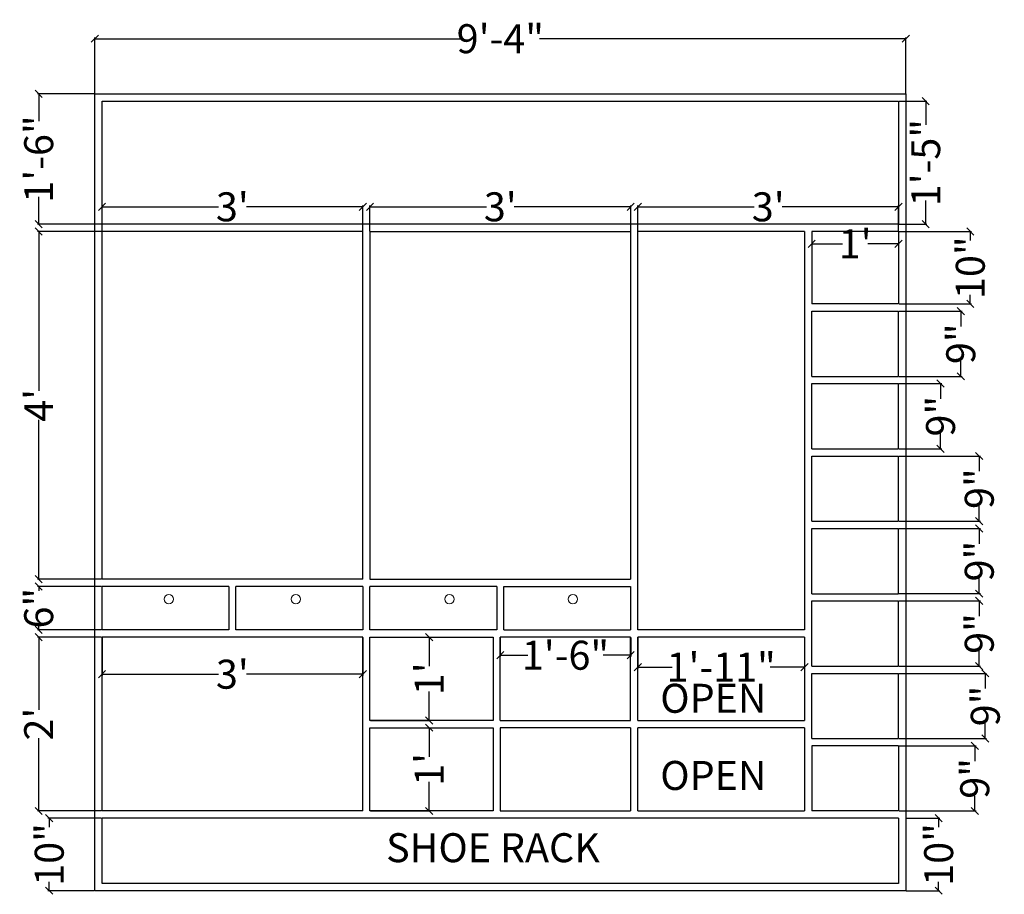
# Model space of a CAD drawing. Units: inches. Extents: x 221 to 357, y 425 to 545.
import ezdxf

# ---------------------------------------------------------------- set-up
doc = ezdxf.new("R2010")
doc.units = ezdxf.units.IN
doc.header["$MEASUREMENT"] = 0
for name, color, linetype, lineweight in [('A-ANNO-DIMS', 2, 'Continuous', 18), ('A-ANNO-TEXT', 3, 'Continuous', 18), ('A-FURN', 7, 'Continuous', 25), ('A-FURN-HDWR', 8, 'Continuous', 13)]:
    doc.layers.add(name, color=color, linetype=linetype, lineweight=lineweight)
doc.styles.get("Standard").update_dxf_attribs({"font": 'arial.ttf'})
doc.dimstyles.get("Standard").update_dxf_attribs({"dimtxt": 4, "dimasz": 1, "dimexe": 0.18, "dimexo": 0.0625, "dimgap": 0.09, "dimtad": 0, "dimdec": 4, "dimzin": 0, "dimdsep": 46, "dimlunit": 4, "dimtxsty": 'Standard', "dimblk": 'OBLIQUE', "dimcen": 0.09, "dimadec": 0, "dimazin": 0, "dimtfac": 1, "dimtdec": 4, "dimtofl": 0, "dimtmove": 0, "dimatfit": 3, "dimldrblk": 'OBLIQUE', "dimfxl": 1, "dimtolj": 1, "dimtzin": 0, "dimarcsym": 1})

# ---------------------------------------------------------------- blocks, each defined once
blk = doc.blocks.new('_Oblique')
at = {"color": 0, "linetype": 'ByBlock', "lineweight": -2}
blk.add_line((-0.5, -0.5), (0.5, 0.5), dxfattribs=at)
blk = doc.blocks.new('*D2')
at = {"layer": 'A-ANNO-DIMS', "color": 0, "lineweight": -2, "transparency": 16777216}
for p, q in [((342.92, 534.06), (346.78, 534.06)), ((346.6, 534.06), (346.6, 530.78)), ((346.6, 517.06), (346.6, 520.34)), ((342.92, 517.06), (346.78, 517.06))]:
    blk.add_line(p, q, dxfattribs=at)
at = {"layer": 'Defpoints', "color": 0, "transparency": 16777216}
for p in [(342.86, 534.06), (342.86, 517.06), (346.6, 517.06)]:
    blk.add_point(p, dxfattribs=at)
at = {"layer": 'A-ANNO-DIMS', "color": 0, "lineweight": -2, "transparency": 16777216}
for p, rotation in [((346.6, 534.06), 90), ((346.6, 517.06), 270)]:
    blk.add_blockref('_Oblique', p, dxfattribs=dict(at, rotation=rotation))
at = {"layer": 'A-ANNO-DIMS', "color": 0, "transparency": 16777216, "insert": (346.6, 525.56), "char_height": 4, "attachment_point": 5, "rotation": 90}
blk.add_mtext('\\A1;1\'-5"', dxfattribs=at)
blk = doc.blocks.new('*D3')
at = {"layer": 'A-ANNO-DIMS', "color": 0, "lineweight": -2, "transparency": 16777216}
for p, q in [((343.92, 435.06), (348.57, 435.06)), ((348.39, 435.06), (348.39, 433.81)), ((348.39, 425.06), (348.39, 426.3)), ((343.92, 425.06), (348.57, 425.06))]:
    blk.add_line(p, q, dxfattribs=at)
at = {"layer": 'Defpoints', "color": 0, "transparency": 16777216}
for p in [(343.86, 435.06), (348.39, 435.06), (343.86, 425.06)]:
    blk.add_point(p, dxfattribs=at)
at = {"layer": 'A-ANNO-DIMS', "color": 0, "lineweight": -2, "transparency": 16777216}
for p, rotation in [((348.39, 435.06), 90), ((348.39, 425.06), 270)]:
    blk.add_blockref('_Oblique', p, dxfattribs=dict(at, rotation=rotation))
at = {"layer": 'A-ANNO-DIMS', "color": 0, "transparency": 16777216, "insert": (348.39, 430.06), "char_height": 4, "attachment_point": 5, "rotation": 90}
blk.add_mtext('\\A1;10"', dxfattribs=at)
blk = doc.blocks.new('*D4')
at = {"layer": 'A-ANNO-DIMS', "color": 0, "lineweight": -2, "transparency": 16777216}
for p, q in [((342.92, 516.06), (352.94, 516.06)), ((352.76, 516.06), (352.76, 514.81)), ((352.76, 506.06), (352.76, 507.3)), ((342.92, 506.06), (352.94, 506.06))]:
    blk.add_line(p, q, dxfattribs=at)
at = {"layer": 'Defpoints', "color": 0, "transparency": 16777216}
for p in [(342.86, 516.06), (342.86, 506.06), (352.76, 506.06)]:
    blk.add_point(p, dxfattribs=at)
at = {"layer": 'A-ANNO-DIMS', "color": 0, "lineweight": -2, "transparency": 16777216}
for p, rotation in [((352.76, 516.06), 90), ((352.76, 506.06), 270)]:
    blk.add_blockref('_Oblique', p, dxfattribs=dict(at, rotation=rotation))
at = {"layer": 'A-ANNO-DIMS', "color": 0, "transparency": 16777216, "insert": (352.76, 511.06), "char_height": 4, "attachment_point": 5, "rotation": 90}
blk.add_mtext('\\A1;10"', dxfattribs=at)
blk = doc.blocks.new('*D5')
at = {"layer": 'A-ANNO-DIMS', "color": 0, "lineweight": -2, "transparency": 16777216}
for p, q in [((342.92, 505.06), (351.62, 505.06)), ((351.44, 505.06), (351.44, 502.95)), ((351.44, 496.06), (351.44, 498.17)), ((342.92, 496.06), (351.62, 496.06))]:
    blk.add_line(p, q, dxfattribs=at)
at = {"layer": 'Defpoints', "color": 0, "transparency": 16777216}
for p in [(342.86, 505.06), (342.86, 496.06), (351.44, 496.06)]:
    blk.add_point(p, dxfattribs=at)
at = {"layer": 'A-ANNO-DIMS', "color": 0, "lineweight": -2, "transparency": 16777216}
for p, rotation in [((351.44, 505.06), 90), ((351.44, 496.06), 270)]:
    blk.add_blockref('_Oblique', p, dxfattribs=dict(at, rotation=rotation))
at = {"layer": 'A-ANNO-DIMS', "color": 0, "transparency": 16777216, "insert": (351.44, 500.56), "char_height": 4, "attachment_point": 5, "rotation": 90}
blk.add_mtext('\\A1;9"', dxfattribs=at)
blk = doc.blocks.new('*D6')
at = {"layer": 'A-ANNO-DIMS', "color": 0, "lineweight": -2, "transparency": 16777216}
for p, q in [((342.92, 495.06), (348.83, 495.06)), ((348.65, 495.06), (348.65, 492.95)), ((348.65, 486.06), (348.65, 488.17)), ((342.92, 486.06), (348.83, 486.06))]:
    blk.add_line(p, q, dxfattribs=at)
at = {"layer": 'Defpoints', "color": 0, "transparency": 16777216}
for p in [(342.86, 495.06), (342.86, 486.06), (348.65, 486.06)]:
    blk.add_point(p, dxfattribs=at)
at = {"layer": 'A-ANNO-DIMS', "color": 0, "lineweight": -2, "transparency": 16777216}
for p, rotation in [((348.65, 495.06), 90), ((348.65, 486.06), 270)]:
    blk.add_blockref('_Oblique', p, dxfattribs=dict(at, rotation=rotation))
at = {"layer": 'A-ANNO-DIMS', "color": 0, "transparency": 16777216, "insert": (348.65, 490.56), "char_height": 4, "attachment_point": 5, "rotation": 90}
blk.add_mtext('\\A1;9"', dxfattribs=at)
blk = doc.blocks.new('*D7')
at = {"layer": 'A-ANNO-DIMS', "color": 0, "lineweight": -2, "transparency": 16777216}
for p, q in [((342.92, 485.06), (354.18, 485.06)), ((354, 485.06), (354, 482.95)), ((354, 476.06), (354, 478.17)), ((342.92, 476.06), (354.18, 476.06))]:
    blk.add_line(p, q, dxfattribs=at)
at = {"layer": 'Defpoints', "color": 0, "transparency": 16777216}
for p in [(342.86, 485.06), (342.86, 476.06), (354, 476.06)]:
    blk.add_point(p, dxfattribs=at)
at = {"layer": 'A-ANNO-DIMS', "color": 0, "lineweight": -2, "transparency": 16777216}
for p, rotation in [((354, 485.06), 90), ((354, 476.06), 270)]:
    blk.add_blockref('_Oblique', p, dxfattribs=dict(at, rotation=rotation))
at = {"layer": 'A-ANNO-DIMS', "color": 0, "transparency": 16777216, "insert": (354, 480.56), "char_height": 4, "attachment_point": 5, "rotation": 90}
blk.add_mtext('\\A1;9"', dxfattribs=at)
blk = doc.blocks.new('*D8')
at = {"layer": 'A-ANNO-DIMS', "color": 0, "lineweight": -2, "transparency": 16777216}
for p, q in [((342.92, 475.06), (354.18, 475.06)), ((354, 475.06), (354, 472.95)), ((354, 466.06), (354, 468.17)), ((342.92, 466.06), (354.18, 466.06))]:
    blk.add_line(p, q, dxfattribs=at)
at = {"layer": 'Defpoints', "color": 0, "transparency": 16777216}
for p in [(342.86, 475.06), (342.86, 466.06), (354, 466.06)]:
    blk.add_point(p, dxfattribs=at)
at = {"layer": 'A-ANNO-DIMS', "color": 0, "lineweight": -2, "transparency": 16777216}
for p, rotation in [((354, 475.06), 90), ((354, 466.06), 270)]:
    blk.add_blockref('_Oblique', p, dxfattribs=dict(at, rotation=rotation))
at = {"layer": 'A-ANNO-DIMS', "color": 0, "transparency": 16777216, "insert": (354, 470.56), "char_height": 4, "attachment_point": 5, "rotation": 90}
blk.add_mtext('\\A1;9"', dxfattribs=at)
blk = doc.blocks.new('*D9')
at = {"layer": 'A-ANNO-DIMS', "color": 0, "lineweight": -2, "transparency": 16777216}
for p, q in [((342.92, 465.06), (354.18, 465.06)), ((354, 465.06), (354, 462.95)), ((354, 456.06), (354, 458.17)), ((342.92, 456.06), (354.18, 456.06))]:
    blk.add_line(p, q, dxfattribs=at)
at = {"layer": 'Defpoints', "color": 0, "transparency": 16777216}
for p in [(342.86, 465.06), (342.86, 456.06), (354, 456.06)]:
    blk.add_point(p, dxfattribs=at)
at = {"layer": 'A-ANNO-DIMS', "color": 0, "lineweight": -2, "transparency": 16777216}
for p, rotation in [((354, 465.06), 90), ((354, 456.06), 270)]:
    blk.add_blockref('_Oblique', p, dxfattribs=dict(at, rotation=rotation))
at = {"layer": 'A-ANNO-DIMS', "color": 0, "transparency": 16777216, "insert": (354, 460.56), "char_height": 4, "attachment_point": 5, "rotation": 90}
blk.add_mtext('\\A1;9"', dxfattribs=at)
blk = doc.blocks.new('*D10')
at = {"layer": 'A-ANNO-DIMS', "color": 0, "lineweight": -2, "transparency": 16777216}
for p, q in [((342.92, 455.06), (355.01, 455.06)), ((354.83, 455.06), (354.83, 452.95)), ((354.83, 446.06), (354.83, 448.17)), ((342.92, 446.06), (355.01, 446.06))]:
    blk.add_line(p, q, dxfattribs=at)
at = {"layer": 'Defpoints', "color": 0, "transparency": 16777216}
for p in [(342.86, 455.06), (342.86, 446.06), (354.83, 446.06)]:
    blk.add_point(p, dxfattribs=at)
at = {"layer": 'A-ANNO-DIMS', "color": 0, "lineweight": -2, "transparency": 16777216}
for p, rotation in [((354.83, 455.06), 90), ((354.83, 446.06), 270)]:
    blk.add_blockref('_Oblique', p, dxfattribs=dict(at, rotation=rotation))
at = {"layer": 'A-ANNO-DIMS', "color": 0, "transparency": 16777216, "insert": (354.83, 450.56), "char_height": 4, "attachment_point": 5, "rotation": 90}
blk.add_mtext('\\A1;9"', dxfattribs=at)
blk = doc.blocks.new('*D11')
at = {"layer": 'A-ANNO-DIMS', "color": 0, "lineweight": -2, "transparency": 16777216}
for p, q in [((342.92, 445.06), (353.55, 445.06)), ((353.37, 445.06), (353.37, 442.95)), ((353.37, 436.06), (353.37, 438.17)), ((342.92, 436.06), (353.55, 436.06))]:
    blk.add_line(p, q, dxfattribs=at)
at = {"layer": 'Defpoints', "color": 0, "transparency": 16777216}
for p in [(342.86, 445.06), (342.86, 436.06), (353.37, 436.06)]:
    blk.add_point(p, dxfattribs=at)
at = {"layer": 'A-ANNO-DIMS', "color": 0, "lineweight": -2, "transparency": 16777216}
for p, rotation in [((353.37, 445.06), 90), ((353.37, 436.06), 270)]:
    blk.add_blockref('_Oblique', p, dxfattribs=dict(at, rotation=rotation))
at = {"layer": 'A-ANNO-DIMS', "color": 0, "transparency": 16777216, "insert": (353.37, 440.56), "char_height": 4, "attachment_point": 5, "rotation": 90}
blk.add_mtext('\\A1;9"', dxfattribs=at)
blk = doc.blocks.new('*D12')
at = {"layer": 'A-ANNO-DIMS', "color": 0, "lineweight": -2, "transparency": 16777216}
for p, q in [((306.86, 460), (306.86, 455.75)), ((329.86, 460), (329.86, 455.75)), ((306.86, 455.93), (311.58, 455.93)), ((329.86, 455.93), (325.13, 455.93))]:
    blk.add_line(p, q, dxfattribs=at)
at = {"layer": 'Defpoints', "color": 0, "transparency": 16777216}
for p in [(306.86, 460.06), (329.86, 460.06), (306.86, 455.93)]:
    blk.add_point(p, dxfattribs=at)
at = {"layer": 'A-ANNO-DIMS', "color": 0, "lineweight": -2, "transparency": 16777216, "rotation": 180}
blk.add_blockref('_Oblique', (306.86, 455.93), dxfattribs=at)
at = {"layer": 'A-ANNO-DIMS', "color": 0, "lineweight": -2, "transparency": 16777216}
blk.add_blockref('_Oblique', (329.86, 455.93), dxfattribs=at)
at = {"layer": 'A-ANNO-DIMS', "color": 0, "transparency": 16777216, "insert": (318.36, 455.93), "char_height": 4, "attachment_point": 5}
blk.add_mtext('\\A1;1\'-11"', dxfattribs=at)
blk = doc.blocks.new('*D13')
at = {"layer": 'A-ANNO-DIMS', "color": 0, "lineweight": -2, "transparency": 16777216}
for p, q in [((287.86, 460), (287.86, 457.38)), ((305.86, 460), (305.86, 457.38)), ((287.86, 457.56), (291.64, 457.56)), ((305.86, 457.56), (302.07, 457.56))]:
    blk.add_line(p, q, dxfattribs=at)
at = {"layer": 'Defpoints', "color": 0, "transparency": 16777216}
for p in [(287.86, 460.06), (305.86, 460.06), (287.86, 457.56)]:
    blk.add_point(p, dxfattribs=at)
at = {"layer": 'A-ANNO-DIMS', "color": 0, "lineweight": -2, "transparency": 16777216, "rotation": 180}
blk.add_blockref('_Oblique', (287.86, 457.56), dxfattribs=at)
at = {"layer": 'A-ANNO-DIMS', "color": 0, "lineweight": -2, "transparency": 16777216}
blk.add_blockref('_Oblique', (305.86, 457.56), dxfattribs=at)
at = {"layer": 'A-ANNO-DIMS', "color": 0, "transparency": 16777216, "insert": (296.86, 457.56), "char_height": 4, "attachment_point": 5}
blk.add_mtext('\\A1;1\'-6"', dxfattribs=at)
blk = doc.blocks.new('*D14')
at = {"layer": 'A-ANNO-DIMS', "color": 0, "lineweight": -2, "transparency": 16777216}
for p, q in [((269.92, 460.06), (278.21, 460.06)), ((278.03, 460.06), (278.03, 456.05)), ((278.03, 448.56), (278.03, 452.57)), ((269.92, 448.56), (278.21, 448.56))]:
    blk.add_line(p, q, dxfattribs=at)
at = {"layer": 'Defpoints', "color": 0, "transparency": 16777216}
for p in [(269.86, 460.06), (278.03, 460.06), (269.86, 448.56)]:
    blk.add_point(p, dxfattribs=at)
at = {"layer": 'A-ANNO-DIMS', "color": 0, "lineweight": -2, "transparency": 16777216}
for p, rotation in [((278.03, 460.06), 90), ((278.03, 448.56), 270)]:
    blk.add_blockref('_Oblique', p, dxfattribs=dict(at, rotation=rotation))
at = {"layer": 'A-ANNO-DIMS', "color": 0, "transparency": 16777216, "insert": (278.03, 454.31), "char_height": 4, "attachment_point": 5, "rotation": 90}
blk.add_mtext("\\A1;1'", dxfattribs=at)
blk = doc.blocks.new('*D15')
at = {"layer": 'A-ANNO-DIMS', "color": 0, "lineweight": -2, "transparency": 16777216}
for p, q in [((232.86, 460), (232.86, 454.76)), ((268.86, 460), (268.86, 454.76)), ((232.86, 454.94), (248.93, 454.94)), ((268.86, 454.94), (252.79, 454.94))]:
    blk.add_line(p, q, dxfattribs=at)
at = {"layer": 'Defpoints', "color": 0, "transparency": 16777216}
for p in [(232.86, 460.06), (268.86, 460.06), (232.86, 454.94)]:
    blk.add_point(p, dxfattribs=at)
at = {"layer": 'A-ANNO-DIMS', "color": 0, "lineweight": -2, "transparency": 16777216, "rotation": 180}
blk.add_blockref('_Oblique', (232.86, 454.94), dxfattribs=at)
at = {"layer": 'A-ANNO-DIMS', "color": 0, "lineweight": -2, "transparency": 16777216}
blk.add_blockref('_Oblique', (268.86, 454.94), dxfattribs=at)
at = {"layer": 'A-ANNO-DIMS', "color": 0, "transparency": 16777216, "insert": (250.86, 454.94), "char_height": 4, "attachment_point": 5}
blk.add_mtext("\\A1;3'", dxfattribs=at)
blk = doc.blocks.new('*D16')
at = {"layer": 'A-ANNO-DIMS', "color": 0, "lineweight": -2, "transparency": 16777216}
for p, q in [((232.86, 516.12), (232.86, 519.64)), ((232.86, 519.46), (248.93, 519.46)), ((268.86, 519.46), (252.79, 519.46)), ((268.86, 516.12), (268.86, 519.64))]:
    blk.add_line(p, q, dxfattribs=at)
at = {"layer": 'Defpoints', "color": 0, "transparency": 16777216}
for p in [(232.86, 519.46), (232.86, 516.06), (268.86, 516.06)]:
    blk.add_point(p, dxfattribs=at)
at = {"layer": 'A-ANNO-DIMS', "color": 0, "lineweight": -2, "transparency": 16777216, "rotation": 180}
blk.add_blockref('_Oblique', (232.86, 519.46), dxfattribs=at)
at = {"layer": 'A-ANNO-DIMS', "color": 0, "lineweight": -2, "transparency": 16777216}
blk.add_blockref('_Oblique', (268.86, 519.46), dxfattribs=at)
at = {"layer": 'A-ANNO-DIMS', "color": 0, "transparency": 16777216, "insert": (250.86, 519.46), "char_height": 4, "attachment_point": 5}
blk.add_mtext("\\A1;3'", dxfattribs=at)
blk = doc.blocks.new('*D17')
at = {"layer": 'A-ANNO-DIMS', "color": 0, "lineweight": -2, "transparency": 16777216}
for p, q in [((269.86, 516.12), (269.86, 519.64)), ((269.86, 519.46), (285.93, 519.46)), ((305.86, 519.46), (289.79, 519.46)), ((305.86, 516.12), (305.86, 519.64))]:
    blk.add_line(p, q, dxfattribs=at)
at = {"layer": 'Defpoints', "color": 0, "transparency": 16777216}
for p in [(269.86, 519.46), (269.86, 516.06), (305.86, 516.06)]:
    blk.add_point(p, dxfattribs=at)
at = {"layer": 'A-ANNO-DIMS', "color": 0, "lineweight": -2, "transparency": 16777216, "rotation": 180}
blk.add_blockref('_Oblique', (269.86, 519.46), dxfattribs=at)
at = {"layer": 'A-ANNO-DIMS', "color": 0, "lineweight": -2, "transparency": 16777216}
blk.add_blockref('_Oblique', (305.86, 519.46), dxfattribs=at)
at = {"layer": 'A-ANNO-DIMS', "color": 0, "transparency": 16777216, "insert": (287.86, 519.46), "char_height": 4, "attachment_point": 5}
blk.add_mtext("\\A1;3'", dxfattribs=at)
blk = doc.blocks.new('*D18')
at = {"layer": 'A-ANNO-DIMS', "color": 0, "lineweight": -2, "transparency": 16777216}
for p, q in [((306.86, 516.12), (306.86, 519.64)), ((306.86, 519.46), (322.93, 519.46)), ((342.86, 519.46), (326.79, 519.46)), ((342.86, 516.12), (342.86, 519.64))]:
    blk.add_line(p, q, dxfattribs=at)
at = {"layer": 'Defpoints', "color": 0, "transparency": 16777216}
for p in [(342.86, 519.46), (306.86, 516.06), (342.86, 516.06)]:
    blk.add_point(p, dxfattribs=at)
at = {"layer": 'A-ANNO-DIMS', "color": 0, "lineweight": -2, "transparency": 16777216, "rotation": 180}
blk.add_blockref('_Oblique', (306.86, 519.46), dxfattribs=at)
at = {"layer": 'A-ANNO-DIMS', "color": 0, "lineweight": -2, "transparency": 16777216}
blk.add_blockref('_Oblique', (342.86, 519.46), dxfattribs=at)
at = {"layer": 'A-ANNO-DIMS', "color": 0, "transparency": 16777216, "insert": (324.86, 519.46), "char_height": 4, "attachment_point": 5}
blk.add_mtext("\\A1;3'", dxfattribs=at)
blk = doc.blocks.new('*D19')
at = {"layer": 'A-ANNO-DIMS', "color": 0, "lineweight": -2, "transparency": 16777216}
for p, q in [((330.86, 516), (330.86, 514.18)), ((342.86, 516), (342.86, 514.18)), ((330.86, 514.36), (335.11, 514.36)), ((342.86, 514.36), (338.6, 514.36))]:
    blk.add_line(p, q, dxfattribs=at)
at = {"layer": 'Defpoints', "color": 0, "transparency": 16777216}
for p in [(330.86, 516.06), (342.86, 516.06), (330.86, 514.36)]:
    blk.add_point(p, dxfattribs=at)
at = {"layer": 'A-ANNO-DIMS', "color": 0, "lineweight": -2, "transparency": 16777216, "rotation": 180}
blk.add_blockref('_Oblique', (330.86, 514.36), dxfattribs=at)
at = {"layer": 'A-ANNO-DIMS', "color": 0, "lineweight": -2, "transparency": 16777216}
blk.add_blockref('_Oblique', (342.86, 514.36), dxfattribs=at)
at = {"layer": 'A-ANNO-DIMS', "color": 0, "transparency": 16777216, "insert": (336.86, 514.36), "char_height": 4, "attachment_point": 5}
blk.add_mtext("\\A1;1'", dxfattribs=at)
blk = doc.blocks.new('*D20')
at = {"layer": 'A-ANNO-DIMS', "color": 0, "lineweight": -2, "transparency": 16777216}
for p, q in [((269.92, 447.56), (278.21, 447.56)), ((278.03, 447.56), (278.03, 443.55)), ((278.03, 436.06), (278.03, 440.07)), ((269.92, 436.06), (278.21, 436.06))]:
    blk.add_line(p, q, dxfattribs=at)
at = {"layer": 'Defpoints', "color": 0, "transparency": 16777216}
for p in [(269.86, 447.56), (278.03, 447.56), (269.86, 436.06)]:
    blk.add_point(p, dxfattribs=at)
at = {"layer": 'A-ANNO-DIMS', "color": 0, "lineweight": -2, "transparency": 16777216}
for p, rotation in [((278.03, 447.56), 90), ((278.03, 436.06), 270)]:
    blk.add_blockref('_Oblique', p, dxfattribs=dict(at, rotation=rotation))
at = {"layer": 'A-ANNO-DIMS', "color": 0, "transparency": 16777216, "insert": (278.03, 441.81), "char_height": 4, "attachment_point": 5, "rotation": 90}
blk.add_mtext("\\A1;1'", dxfattribs=at)
blk = doc.blocks.new('*D21')
at = {"layer": 'A-ANNO-DIMS', "color": 0, "lineweight": -2, "transparency": 16777216}
for p, q in [((232.79, 435.06), (225.39, 435.06)), ((225.57, 435.06), (225.57, 433.81)), ((225.57, 425.06), (225.57, 426.3)), ((231.79, 425.06), (225.39, 425.06))]:
    blk.add_line(p, q, dxfattribs=at)
at = {"layer": 'Defpoints', "color": 0, "transparency": 16777216}
for p in [(225.57, 435.06), (232.86, 435.06), (231.86, 425.06)]:
    blk.add_point(p, dxfattribs=at)
at = {"layer": 'A-ANNO-DIMS', "color": 0, "lineweight": -2, "transparency": 16777216}
for p, rotation in [((225.57, 435.06), 90), ((225.57, 425.06), 270)]:
    blk.add_blockref('_Oblique', p, dxfattribs=dict(at, rotation=rotation))
at = {"layer": 'A-ANNO-DIMS', "color": 0, "transparency": 16777216, "insert": (225.57, 430.06), "char_height": 4, "attachment_point": 5, "rotation": 90}
blk.add_mtext('\\A1;10"', dxfattribs=at)
blk = doc.blocks.new('*D22')
at = {"layer": 'A-ANNO-DIMS', "color": 0, "lineweight": -2, "transparency": 16777216}
for p, q in [((232.79, 460.06), (223.93, 460.06)), ((224.11, 460.06), (224.11, 450.02)), ((224.11, 436.06), (224.11, 446.09)), ((232.79, 436.06), (223.93, 436.06))]:
    blk.add_line(p, q, dxfattribs=at)
at = {"layer": 'Defpoints', "color": 0, "transparency": 16777216}
for p in [(224.11, 460.06), (232.86, 460.06), (232.86, 436.06)]:
    blk.add_point(p, dxfattribs=at)
at = {"layer": 'A-ANNO-DIMS', "color": 0, "lineweight": -2, "transparency": 16777216}
for p, rotation in [((224.11, 460.06), 90), ((224.11, 436.06), 270)]:
    blk.add_blockref('_Oblique', p, dxfattribs=dict(at, rotation=rotation))
at = {"layer": 'A-ANNO-DIMS', "color": 0, "transparency": 16777216, "insert": (224.11, 448.06), "char_height": 4, "attachment_point": 5, "rotation": 90}
blk.add_mtext("\\A1;2'", dxfattribs=at)
blk = doc.blocks.new('*D23')
at = {"layer": 'A-ANNO-DIMS', "color": 0, "lineweight": -2, "transparency": 16777216}
for p, q in [((232.79, 467.06), (223.93, 467.06)), ((224.11, 467.06), (224.11, 466.46)), ((232.79, 461.06), (223.93, 461.06)), ((224.11, 461.06), (224.11, 461.66))]:
    blk.add_line(p, q, dxfattribs=at)
at = {"layer": 'Defpoints', "color": 0, "transparency": 16777216}
for p in [(224.11, 467.06), (232.86, 467.06), (232.86, 461.06)]:
    blk.add_point(p, dxfattribs=at)
at = {"layer": 'A-ANNO-DIMS', "color": 0, "lineweight": -2, "transparency": 16777216}
for p, rotation in [((224.11, 467.06), 90), ((224.11, 461.06), 270)]:
    blk.add_blockref('_Oblique', p, dxfattribs=dict(at, rotation=rotation))
at = {"layer": 'A-ANNO-DIMS', "color": 0, "transparency": 16777216, "insert": (224.11, 464.06), "char_height": 4, "attachment_point": 5, "rotation": 90}
blk.add_mtext('\\A1;6"', dxfattribs=at)
blk = doc.blocks.new('*D24')
at = {"layer": 'A-ANNO-DIMS', "color": 0, "lineweight": -2, "transparency": 16777216}
for p, q in [((232.79, 516.06), (223.93, 516.06)), ((224.11, 516.06), (224.11, 494.07)), ((224.11, 468.06), (224.11, 490.05)), ((232.79, 468.06), (223.93, 468.06))]:
    blk.add_line(p, q, dxfattribs=at)
at = {"layer": 'Defpoints', "color": 0, "transparency": 16777216}
for p in [(224.11, 516.06), (232.86, 516.06), (232.86, 468.06)]:
    blk.add_point(p, dxfattribs=at)
at = {"layer": 'A-ANNO-DIMS', "color": 0, "lineweight": -2, "transparency": 16777216}
for p, rotation in [((224.11, 516.06), 90), ((224.11, 468.06), 270)]:
    blk.add_blockref('_Oblique', p, dxfattribs=dict(at, rotation=rotation))
at = {"layer": 'A-ANNO-DIMS', "color": 0, "transparency": 16777216, "insert": (224.11, 492.06), "char_height": 4, "attachment_point": 5, "rotation": 90}
blk.add_mtext("\\A1;4'", dxfattribs=at)
blk = doc.blocks.new('*D25')
at = {"layer": 'A-ANNO-DIMS', "color": 0, "lineweight": -2, "transparency": 16777216}
for p, q in [((231.79, 535.06), (223.93, 535.06)), ((224.11, 535.06), (224.11, 531.28)), ((224.11, 517.06), (224.11, 520.84)), ((232.79, 517.06), (223.93, 517.06))]:
    blk.add_line(p, q, dxfattribs=at)
at = {"layer": 'Defpoints', "color": 0, "transparency": 16777216}
for p in [(231.86, 535.06), (224.11, 517.06), (232.86, 517.06)]:
    blk.add_point(p, dxfattribs=at)
at = {"layer": 'A-ANNO-DIMS', "color": 0, "lineweight": -2, "transparency": 16777216}
for p, rotation in [((224.11, 535.06), 90), ((224.11, 517.06), 270)]:
    blk.add_blockref('_Oblique', p, dxfattribs=dict(at, rotation=rotation))
at = {"layer": 'A-ANNO-DIMS', "color": 0, "transparency": 16777216, "insert": (224.11, 526.06), "char_height": 4, "attachment_point": 5, "rotation": 90}
blk.add_mtext('\\A1;1\'-6"', dxfattribs=at)
blk = doc.blocks.new('*D26')
at = {"layer": 'A-ANNO-DIMS', "color": 0, "lineweight": -2, "transparency": 16777216}
for p, q in [((231.86, 535.12), (231.86, 542.85)), ((231.86, 542.67), (282.45, 542.67)), ((343.86, 542.67), (293.26, 542.67)), ((343.86, 535.12), (343.86, 542.85))]:
    blk.add_line(p, q, dxfattribs=at)
at = {"layer": 'Defpoints', "color": 0, "transparency": 16777216}
for p in [(343.86, 542.67), (231.86, 535.06), (343.86, 535.06)]:
    blk.add_point(p, dxfattribs=at)
at = {"layer": 'A-ANNO-DIMS', "color": 0, "lineweight": -2, "transparency": 16777216, "rotation": 180}
blk.add_blockref('_Oblique', (231.86, 542.67), dxfattribs=at)
at = {"layer": 'A-ANNO-DIMS', "color": 0, "lineweight": -2, "transparency": 16777216}
blk.add_blockref('_Oblique', (343.86, 542.67), dxfattribs=at)
at = {"layer": 'A-ANNO-DIMS', "color": 0, "transparency": 16777216, "insert": (287.86, 542.67), "char_height": 4, "attachment_point": 5}
blk.add_mtext('\\A1;9\'-4"', dxfattribs=at)
blk = doc.blocks.new('SHELF-CUBBY')
for p, q in [((12, 9), (0, 9)), ((0, 9), (0, 0)), ((12, 9), (12, 0)), ((12, 0), (0, 0))]:
    blk.add_line(p, q)
blk = doc.blocks.new('DRAWER-FRONT')
for p, q in [((0, 0), (0, 6)), ((17.5, 6), (0, 6)), ((17.5, 6), (17.5, 0)), ((17.5, 0), (0, 0))]:
    blk.add_line(p, q)
blk = doc.blocks.new('SHUTTER-HANGING')
for p, q in [((0, 0), (0, 48)), ((36, 48), (0, 48)), ((36, 0), (36, 48)), ((36, 0), (0, 0))]:
    blk.add_line(p, q)
blk = doc.blocks.new('SHOE-RACK-BAY')
for p, q in [((23, 11.5), (0, 11.5)), ((0, 0), (0, 11.5)), ((23, 11.5), (23, 0)), ((0, 0), (23, 0))]:
    blk.add_line(p, q)
blk = doc.blocks.new('SHELF-BAY-A')
for p, q in [((18, 11.5), (0, 11.5)), ((0, 0), (0, 11.5)), ((18, 0), (18, 11.5)), ((0, 0), (18, 0))]:
    blk.add_line(p, q)
blk = doc.blocks.new('SHELF-BAY-B')
for p, q in [((0, 0), (0, 11.5)), ((0, 11.5), (17, 11.5)), ((17, 11.5), (17, 0)), ((17, 0), (0, 0))]:
    blk.add_line(p, q)

msp = doc.modelspace()

# ---------------------------------------------------------------- linework, layer by layer
at = {"layer": 'A-FURN'}
for p, q in [((231.85672, 535.05911), (343.85672, 535.05911)), ((231.85672, 425.05911), (231.85672, 535.05911)), ((343.85672, 535.05911), (343.85672, 517.05911)), ((232.85672, 534.05911), (342.85672, 534.05911)), ((232.85672, 517.05911), (232.85672, 534.05911)), ((342.85672, 534.05911), (342.85672, 517.05911)), ((342.85672, 517.05911), (232.85672, 517.05911)), ((343.85672, 517.05911), (343.85672, 516.05911)), ((306.85672, 467.05911), (306.85672, 516.05911)), ((329.85672, 516.05911), (306.85672, 516.05911)), ((329.85672, 516.05911), (329.85672, 461.05911)), ((342.85672, 516.05911), (330.85672, 516.05911)), ((330.85672, 516.05911), (330.85672, 506.05911)), ((342.85672, 516.05911), (342.85672, 506.05911)), ((343.85672, 516.05911), (343.85672, 468.05911)), ((342.85672, 506.05911), (330.85672, 506.05911)), ((343.85672, 468.05911), (343.85672, 467.05911)), ((306.85672, 461.05911), (306.85672, 467.05911)), ((343.85672, 467.05911), (343.85672, 461.05911)), ((329.85672, 461.05911), (306.85672, 461.05911)), ((343.85672, 461.05911), (343.85672, 460.05911)), ((232.85672, 436.05911), (232.85672, 460.05911)), ((268.85672, 460.05911), (232.85672, 460.05911)), ((268.85672, 436.05911), (268.85672, 460.05911)), ((343.85672, 460.05911), (343.85672, 436.05911)), ((268.85672, 436.05911), (232.85672, 436.05911)), ((343.85672, 436.05911), (343.85672, 435.05911)), ((232.85672, 426.05911), (232.85672, 435.05911)), ((342.85672, 435.05911), (232.85672, 435.05911)), ((342.85672, 435.05911), (342.85672, 426.05911)), ((343.85672, 435.05911), (343.85672, 425.05911)), ((342.85672, 426.05911), (232.85672, 426.05911)), ((343.85672, 425.05911), (231.85672, 425.05911))]:
    msp.add_line(p, q, dxfattribs=at)
at = {"layer": 'A-FURN-HDWR'}
for centre in [(242.0846, 465.29933), (259.625, 465.29933), (280.8323, 465.29933), (297.87921, 465.29933)]:
    msp.add_circle(centre, 0.63902, dxfattribs=at)

# ---------------------------------------------------------------- block references
at = {"layer": 'A-FURN'}
for name, p in [('SHUTTER-HANGING', (232.857, 468.059)), ('DRAWER-FRONT', (232.857, 461.059)), ('DRAWER-FRONT', (251.357, 461.059)), ('DRAWER-FRONT', (269.857, 461.059)), ('SHELF-BAY-A', (287.857, 448.559)), ('SHOE-RACK-BAY', (306.857, 448.559)), ('SHELF-BAY-B', (269.857, 436.059)), ('SHELF-CUBBY', (330.857, 436.059))]:
    msp.add_blockref(name, p, dxfattribs=at)
at = {"layer": 'A-FURN', "rotation": 180}
for name, p in [('SHUTTER-HANGING', (305.85643, 516.05923)), ('SHELF-CUBBY', (342.85643, 505.05923)), ('SHELF-CUBBY', (342.85643, 495.05923)), ('SHELF-CUBBY', (342.85643, 485.05923)), ('SHELF-CUBBY', (342.85643, 475.05923)), ('DRAWER-FRONT', (305.85643, 467.05923)), ('SHELF-CUBBY', (342.85643, 465.05923)), ('SHELF-BAY-B', (286.85643, 460.05923)), ('SHELF-CUBBY', (342.85643, 455.05923)), ('SHELF-BAY-A', (305.85643, 447.55923)), ('SHOE-RACK-BAY', (329.85643, 447.55923))]:
    msp.add_blockref(name, p, dxfattribs=at)

# ---------------------------------------------------------------- texts
at = {"layer": 'A-ANNO-TEXT', "char_height": 4, "attachment_point": 1}
for s, width, insert in [('OPEN', 16.4799889, (309.95033, 453.61721)), ('OPEN', 16.4799889, (309.95033, 442.96647)), ('\\pxqc;SHOE RACK', 47.2576811, (263.21244, 432.99129))]:
    msp.add_mtext_dynamic_manual_height_columns(s, width=width, gutter_width=20, heights=[0], dxfattribs=dict(at, insert=insert))

# ---------------------------------------------------------------- dimensions: what is measured, and where the dimension line sits
at = {"layer": 'A-ANNO-DIMS'}
for base, p1, p2, picture, middle in [((343.85672, 542.66716), (231.85672, 535.05911), (343.85672, 535.05911), '*D26', (287.85672, 542.66716)), ((232.85672, 519.46168), (268.85672, 516.05911), (232.85672, 516.05911), '*D16', (250.85672, 519.46168)), ((269.85672, 519.46168), (305.85672, 516.05911), (269.85672, 516.05911), '*D17', (287.85672, 519.46168)), ((342.85672, 519.46168), (306.85672, 516.05911), (342.85672, 516.05911), '*D18', (324.85672, 519.46168)), ((330.85672, 514.35914), (342.85672, 516.05911), (330.85672, 516.05911), '*D19', (336.85672, 514.35914)), ((232.85672, 454.93719), (268.85672, 460.05911), (232.85672, 460.05911), '*D15', (250.85672, 454.93719)), ((287.85672, 457.56356), (305.85672, 460.05911), (287.85672, 460.05911), '*D13', (296.85672, 457.56356)), ((306.85672, 455.92978), (329.85672, 460.05911), (306.85672, 460.05911), '*D12', (318.35672, 455.92978))]:
    dim = msp.add_linear_dim(base=base, p1=p1, p2=p2, dimstyle='Standard', override={"dimclrd": 0, "dimclre": 0, "dimclrt": 0}, dxfattribs=at)
    dim.commit()
    dim.dimension.update_dxf_attribs({"geometry": picture, "text_midpoint": middle})
for base, p1, p2, picture, middle in [((224.1141, 517.05911), (231.85672, 535.05911), (232.85672, 517.05911), '*D25', (224.1141, 526.05911)), ((346.60113, 517.05911), (342.85672, 534.05911), (342.85672, 517.05911), '*D2', (346.60113, 525.55911)), ((224.1141, 516.05911), (232.85672, 468.05911), (232.85672, 516.05911), '*D24', (224.1141, 492.05911)), ((352.76207, 506.05911), (342.85672, 516.05911), (342.85672, 506.05911), '*D4', (352.76207, 511.05911)), ((351.43952, 496.05911), (342.85672, 505.05911), (342.85672, 496.05911), '*D5', (351.43952, 500.55911)), ((348.6529, 486.05911), (342.85672, 495.05911), (342.85672, 486.05911), '*D6', (348.6529, 490.55911)), ((353.99733, 476.05911), (342.85672, 485.05911), (342.85672, 476.05911), '*D7', (353.99733, 480.55911)), ((353.99733, 466.05911), (342.85672, 475.05911), (342.85672, 466.05911), '*D8', (353.99733, 470.55911)), ((224.1141, 467.05911), (232.85672, 461.05911), (232.85672, 467.05911), '*D23', (224.1141, 464.05911)), ((353.99733, 456.05911), (342.85672, 465.05911), (342.85672, 456.05911), '*D9', (353.99733, 460.55911)), ((224.1141, 460.05911), (232.85672, 436.05911), (232.85672, 460.05911), '*D22', (224.1141, 448.05911)), ((354.83171, 446.05911), (342.85672, 455.05911), (342.85672, 446.05911), '*D10', (354.83171, 450.55911)), ((353.37469, 436.05911), (342.85672, 445.05911), (342.85672, 436.05911), '*D11', (353.37469, 440.55911)), ((225.56506, 435.05911), (231.85672, 425.05911), (232.85672, 435.05911), '*D21', (225.56506, 430.05911)), ((348.38978, 435.05911), (343.85672, 425.05911), (343.85672, 435.05911), '*D3', (348.38978, 430.05911))]:
    dim = msp.add_linear_dim(base=base, p1=p1, p2=p2, angle=90, dimstyle='Standard', override={"dimclrd": 0, "dimclre": 0, "dimclrt": 0}, dxfattribs=at)
    dim.commit()
    dim.dimension.update_dxf_attribs({"geometry": picture, "text_midpoint": middle})
for base, p1, p2, picture, middle in [((278.03405, 460.05911), (269.85672, 448.55911), (269.85672, 460.05911), '*D14', (278.03405, 454.30911)), ((278.03405, 447.55911), (269.85672, 436.05911), (269.85672, 447.55911), '*D20', (278.03405, 441.80911))]:
    dim = msp.add_linear_dim(base=base, p1=p1, p2=p2, angle=90, text="1'", dimstyle='Standard', override={"dimclrd": 0, "dimclre": 0, "dimclrt": 0}, dxfattribs=at)
    dim.commit()
    dim.dimension.update_dxf_attribs({"geometry": picture, "text_midpoint": middle})

doc.saveas('drawing.dxf')
